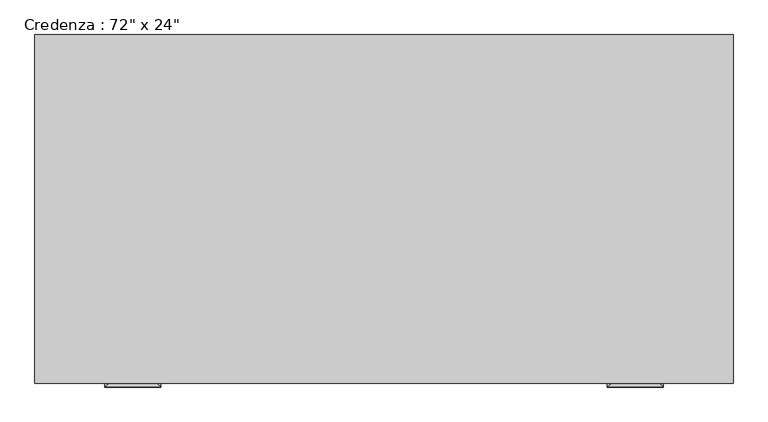
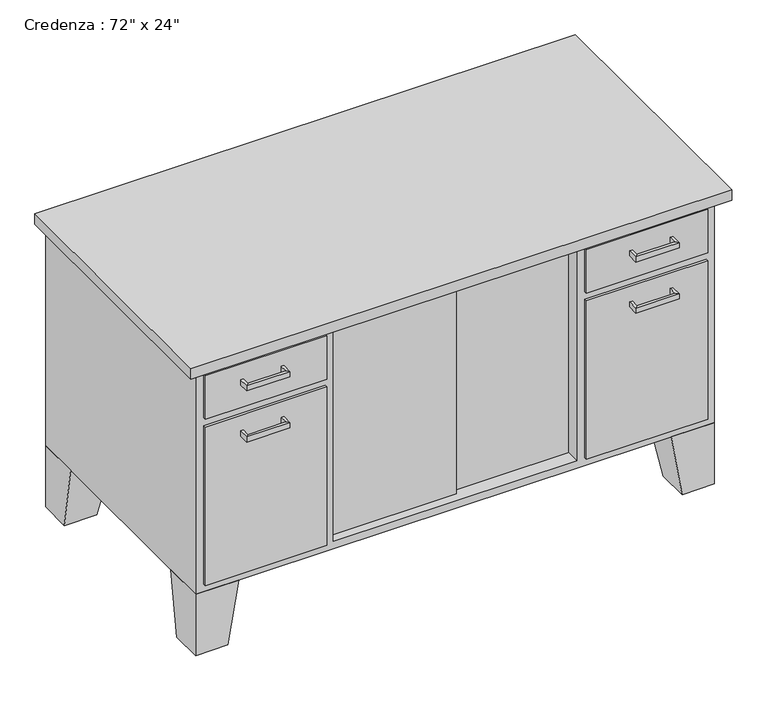
"""IFC4 building model written with IfcOpenShell, lengths in millimetres: furniture geometry."""

from ifc_helpers import new_model, si_unit, frame, origin, place, context, project, spatial, polyline, outline, extrude, faceted_brep, source, transform, mapped, element, save


def furniture_201ebc49(model_context):
    return source(origin(), model_context, "Body", "SolidModel", [
        extrude(outline(polyline([(379.3023176, -267.2714583), (46.8442623, -267.2714583), (46.8442623, -254.5714583), (379.3023176, -254.5714583), (379.3023176, -267.2714583)])), frame((0.0, 0.0, 171.45), z_axis=(0.0, 0.0, 1.0), x_axis=(1.0, 0.0, 0.0)), (0.0, 0.0, 1.0), 520.7),
        extrude(outline(polyline([(73.6254475, -279.9714583), (-226.2057377, -279.9714583), (-226.2057377, -267.2714583), (73.6254475, -267.2714583), (73.6254475, -279.9714583)])), frame((0.0, 0.0, 171.45), z_axis=(0.0, 0.0, 1.0), x_axis=(1.0, 0.0, 0.0)), (0.0, 0.0, 1.0), 520.7),
        faceted_brep([(567.5442623, 309.3803279, 152.4), (567.5442623, 207.7803279, 152.4), (669.1442623, 207.7803279, 152.4), (669.1442623, 309.3803279, 152.4), (592.9442623, 309.3803279, 0.0), (669.1442623, 309.3803279, 0.0), (669.1442623, 233.1803279, 0.0), (592.9442623, 233.1803279, 0.0)], [[[0, 1, 2, 3]], [[4, 5, 6, 7]], [[4, 7, 1, 0]], [[7, 6, 2, 1]], [[6, 5, 3, 2]], [[5, 4, 0, 3]]]),
        extrude(outline(polyline([(650.0942623, -306.5696721), (364.3442623, -306.5696721), (364.3442623, -300.2196721), (650.0942623, -300.2196721), (650.0942623, -306.5696721)])), frame((0.0, 0.0, 584.2), z_axis=(0.0, 0.0, 1.0), x_axis=(1.0, 0.0, 0.0)), (0.0, 0.0, 1.0), 107.95),
        extrude(outline(polyline([(650.0942623, -306.5696721), (364.3442623, -306.5696721), (364.3442623, -300.2196721), (650.0942623, -300.2196721), (650.0942623, -306.5696721)])), frame((0.0, 0.0, 171.45), z_axis=(0.0, 0.0, 1.0), x_axis=(1.0, 0.0, 0.0)), (0.0, 0.0, 1.0), 393.7),
        extrude(outline(polyline([(-245.2557377, -306.5696721), (-531.0057377, -306.5696721), (-531.0057377, -300.2196721), (-245.2557377, -300.2196721), (-245.2557377, -306.5696721)])), frame((0.0, 0.0, 584.2), z_axis=(0.0, 0.0, 1.0), x_axis=(1.0, 0.0, 0.0)), (0.0, 0.0, 1.0), 107.95),
        extrude(outline(polyline([(-245.2557377, -306.5696721), (-531.0057377, -306.5696721), (-531.0057377, -300.2196721), (-245.2557377, -300.2196721), (-245.2557377, -306.5696721)])), frame((0.0, 0.0, 171.45), z_axis=(0.0, 0.0, 1.0), x_axis=(1.0, 0.0, 0.0)), (0.0, 0.0, 1.0), 393.7),
        faceted_brep([(-448.4557377, -300.2196721, 152.4), (-448.4557377, -198.6196721, 152.4), (-550.0557377, -198.6196721, 152.4), (-550.0557377, -300.2196721, 152.4), (-473.8557377, -300.2196721, 0.0), (-550.0557377, -300.2196721, 0.0), (-550.0557377, -224.0196721, 0.0), (-473.8557377, -224.0196721, 0.0)], [[[0, 1, 2, 3]], [[4, 5, 6, 7]], [[4, 7, 1, 0]], [[7, 6, 2, 1]], [[6, 5, 3, 2]], [[5, 4, 0, 3]]]),
        faceted_brep([(-448.4557377, 309.3803279, 152.4), (-550.0557377, 309.3803279, 152.4), (-550.0557377, 207.7803279, 152.4), (-448.4557377, 207.7803279, 152.4), (-473.8557377, 309.3803279, 0.0), (-473.8557377, 233.1803279, 0.0), (-550.0557377, 233.1803279, 0.0), (-550.0557377, 309.3803279, 0.0)], [[[0, 1, 2, 3]], [[4, 5, 6, 7]], [[4, 7, 1, 0]], [[7, 6, 2, 1]], [[6, 5, 3, 2]], [[5, 4, 0, 3]]]),
        faceted_brep([(567.5442623, -300.2196721, 152.4), (669.1442623, -300.2196721, 152.4), (669.1442623, -198.6196721, 152.4), (567.5442623, -198.6196721, 152.4), (592.9442623, -300.2196721, 0.0), (592.9442623, -224.0196721, 0.0), (669.1442623, -224.0196721, 0.0), (669.1442623, -300.2196721, 0.0)], [[[0, 1, 2, 3]], [[4, 5, 6, 7]], [[4, 7, 1, 0]], [[7, 6, 2, 1]], [[6, 5, 3, 2]], [[5, 4, 0, 3]]]),
        faceted_brep([(669.1442623, 309.3803279, 711.2), (-550.0557377, 309.3803279, 711.2), (-550.0557377, -300.2196721, 711.2), (669.1442623, -300.2196721, 711.2), (669.1442623, 309.3803279, 152.4), (669.1442623, -300.2196721, 152.4), (-550.0557377, -300.2196721, 152.4), (-550.0557377, 309.3803279, 152.4), (-226.2057377, -300.2196721, 692.15), (345.2942623, -300.2196721, 692.15), (345.2942623, -300.2196721, 171.45), (-226.2057377, -300.2196721, 171.45), (345.2942623, 290.3303279, 692.15), (-226.2057377, 290.3303279, 692.15), (-226.2057377, 290.3303279, 171.45), (345.2942623, 290.3303279, 171.45)], [[[0, 1, 2, 3]], [[4, 5, 6, 7]], [[1, 0, 4, 7]], [[2, 1, 7, 6]], [[3, 2, 6, 5], [8, 9, 10, 11]], [[0, 3, 5, 4]], [[12, 13, 14, 15]], [[13, 12, 9, 8]], [[14, 13, 8, 11]], [[15, 14, 11, 10]], [[12, 15, 10, 9]]]),
        extrude(outline(polyline([(694.5442623, 309.3803279), (694.5442623, -325.6196721), (-575.4557377, -325.6196721), (-575.4557377, 309.3803279), (694.5442623, 309.3803279)])), frame((0.0, 0.0, 711.2), z_axis=(0.0, 0.0, 1.0), x_axis=(1.0, 0.0, 0.0)), (0.0, 0.0, 1.0), 25.4),
        faceted_brep([(-442.1057377, -306.5696721, 527.05), (-442.1057377, -306.5696721, 514.35), (-448.4557377, -306.5696721, 514.35), (-448.4557377, -306.5696721, 527.05), (-442.1057377, -325.6196721, 527.05), (-442.1057377, -325.6196721, 514.35), (-448.4557377, -331.9696721, 514.35), (-448.4557377, -331.9696721, 527.05), (-353.2057377, -325.6196721, 527.05), (-353.2057377, -325.6196721, 514.35), (-346.8557377, -331.9696721, 514.35), (-346.8557377, -331.9696721, 527.05), (-353.2057377, -306.5696721, 527.05), (-346.8557377, -306.5696721, 527.05), (-346.8557377, -306.5696721, 514.35), (-353.2057377, -306.5696721, 514.35)], [[[0, 1, 2, 3]], [[1, 0, 4, 5]], [[2, 1, 5, 6]], [[3, 2, 6, 7]], [[0, 3, 7, 4]], [[5, 4, 8, 9]], [[6, 5, 9, 10]], [[7, 6, 10, 11]], [[4, 7, 11, 8]], [[12, 13, 14, 15]], [[9, 8, 12, 15]], [[10, 9, 15, 14]], [[11, 10, 14, 13]], [[8, 11, 13, 12]]]),
        faceted_brep([(-442.1057377, -306.5696721, 654.05), (-442.1057377, -306.5696721, 641.35), (-448.4557377, -306.5696721, 641.35), (-448.4557377, -306.5696721, 654.05), (-442.1057377, -325.6196721, 654.05), (-442.1057377, -325.6196721, 641.35), (-448.4557377, -331.9696721, 641.35), (-448.4557377, -331.9696721, 654.05), (-353.2057377, -325.6196721, 654.05), (-353.2057377, -325.6196721, 641.35), (-346.8557377, -331.9696721, 641.35), (-346.8557377, -331.9696721, 654.05), (-353.2057377, -306.5696721, 654.05), (-346.8557377, -306.5696721, 654.05), (-346.8557377, -306.5696721, 641.35), (-353.2057377, -306.5696721, 641.35)], [[[0, 1, 2, 3]], [[1, 0, 4, 5]], [[2, 1, 5, 6]], [[3, 2, 6, 7]], [[0, 3, 7, 4]], [[5, 4, 8, 9]], [[6, 5, 9, 10]], [[7, 6, 10, 11]], [[4, 7, 11, 8]], [[12, 13, 14, 15]], [[9, 8, 12, 15]], [[10, 9, 15, 14]], [[11, 10, 14, 13]], [[8, 11, 13, 12]]]),
        faceted_brep([(472.2942623, -306.5696721, 654.1373112), (472.2942623, -306.5696721, 641.4373112), (465.9442623, -306.5696721, 641.4373112), (465.9442623, -306.5696721, 654.1373112), (472.2942623, -325.6196721, 654.1373112), (472.2942623, -325.6196721, 641.4373112), (465.9442623, -331.9696721, 641.4373112), (465.9442623, -331.9696721, 654.1373112), (561.1942623, -325.6196721, 654.1373112), (561.1942623, -325.6196721, 641.4373112), (567.5442623, -331.9696721, 641.4373112), (567.5442623, -331.9696721, 654.1373112), (561.1942623, -306.5696721, 654.1373112), (567.5442623, -306.5696721, 654.1373112), (567.5442623, -306.5696721, 641.4373112), (561.1942623, -306.5696721, 641.4373112)], [[[0, 1, 2, 3]], [[1, 0, 4, 5]], [[2, 1, 5, 6]], [[3, 2, 6, 7]], [[0, 3, 7, 4]], [[5, 4, 8, 9]], [[6, 5, 9, 10]], [[7, 6, 10, 11]], [[4, 7, 11, 8]], [[12, 13, 14, 15]], [[9, 8, 12, 15]], [[10, 9, 15, 14]], [[11, 10, 14, 13]], [[8, 11, 13, 12]]]),
        faceted_brep([(472.2942623, -306.5696721, 527.05), (472.2942623, -306.5696721, 514.35), (465.9442623, -306.5696721, 514.35), (465.9442623, -306.5696721, 527.05), (472.2942623, -325.6196721, 527.05), (472.2942623, -325.6196721, 514.35), (465.9442623, -331.9696721, 514.35), (465.9442623, -331.9696721, 527.05), (561.1942623, -325.6196721, 527.05), (561.1942623, -325.6196721, 514.35), (567.5442623, -331.9696721, 514.35), (567.5442623, -331.9696721, 527.05), (561.1942623, -306.5696721, 527.05), (567.5442623, -306.5696721, 527.05), (567.5442623, -306.5696721, 514.35), (561.1942623, -306.5696721, 514.35)], [[[0, 1, 2, 3]], [[1, 0, 4, 5]], [[2, 1, 5, 6]], [[3, 2, 6, 7]], [[0, 3, 7, 4]], [[5, 4, 8, 9]], [[6, 5, 9, 10]], [[7, 6, 10, 11]], [[4, 7, 11, 8]], [[12, 13, 14, 15]], [[9, 8, 12, 15]], [[10, 9, 15, 14]], [[11, 10, 14, 13]], [[8, 11, 13, 12]]]),
    ])


if __name__ == "__main__":
    model = new_model("IFC4")
    model_context = context("Model", 3, world=origin())
    ifc_project = project(units=[si_unit("LENGTHUNIT", "METRE", prefix="MILLI")], contexts=[model_context])
    site = spatial("IfcSite", under=ifc_project)
    building = spatial("IfcBuilding", under=site)
    placement = place(None, origin())
    furniture_shape = furniture_201ebc49(model_context)
    element("IfcFurniture", 1, ObjectType="Credenza : 72\" x 24\"", at=placement, inside=building, context=model_context, shape_type="MappedRepresentation", body=[
        mapped(furniture_shape, transform((0.0, 0.0, 0.0), x_axis=(1.0, 0.0, 0.0), y_axis=(0.0, 1.0, 0.0), z_axis=(0.0, 0.0, 1.0))),
    ])
    save(model, "model.ifc")

# Revit data of these elements
# Type "Credenza : 72\" x 24\""
#   Assembly Code = "E2020200"
#   Depth = 2' - 0"
#   Height = 2' - 5"
#   Width = 4' - 0"
#   Body Material = Laminate, Ivory, Matte
#   Handles/Legs Material = Steel, Chrome Plated
#   Top Material = Cherry
#   Default Elevation = 0
# Element 1 (IfcFurniture, "Credenza : 72\" x 24\"")
#   Materials on its faces: "Steel, Chrome Plated", "Laminate, Ivory, Matte", "Cherry"
# Materials
#   "Laminate, Ivory, Matte": class "Plastic", colour RGB 247 247 239, transparency 0, Description = "Plastic Laminate - Ivory, Matte", Cost = 0
#   "Steel, Chrome Plated": class "Metal", colour RGB 17 17 17, transparency 0, Description = "Chromiuim plated steel", Cost = 0
#   "Cherry": class "Wood", colour RGB 226 177 128, transparency 0, Description = "Prunus Serotina", Cost = 0
